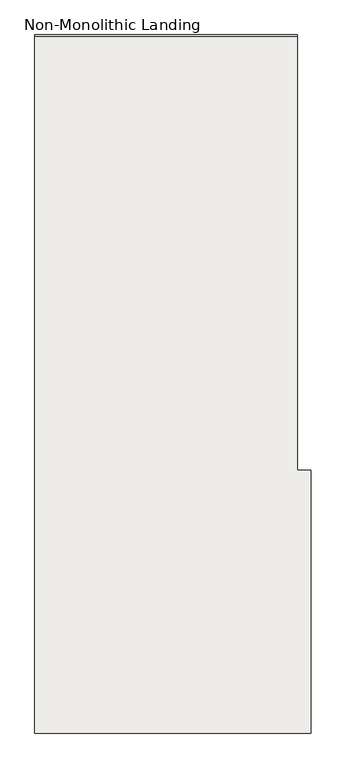
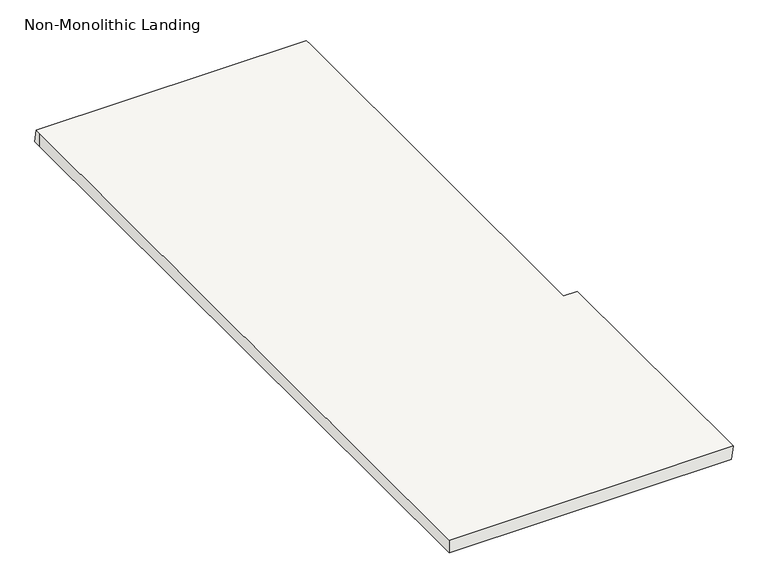
"""IFC4 building model written with IfcOpenShell, lengths in millimetres: slab geometry, Non-Monolithic Landing."""

from ifc_helpers import new_model, si_unit, origin, place, context, project, spatial, faceted_brep, source, transform, mapped, element, save


def non_monolithic_landing_de183352(model_context):
    return source(origin(), model_context, "Body", "Brep", [
        faceted_brep([(-11551.2529994, 5709.8660835, 1043.4782609), (-11602.0529994, 5709.8660835, 1043.4782609), (-11602.0529994, 7333.8660835, 1043.4782609), (-11602.0529994, 7358.8660835, 1043.4782609), (-12602.0787807, 7358.8660835, 1043.4782609), (-12602.0787807, 7333.8660835, 1043.4782609), (-12602.0787807, 4709.8403022, 1043.4782609), (-11551.2529994, 4709.8403022, 1043.4782609), (-11602.0529994, 7333.8660835, 993.4782609), (-11602.0529994, 5709.8660835, 993.4782609), (-11558.4404994, 5709.8660835, 993.4782609), (-11558.4404994, 4709.8403022, 993.4782609), (-12602.0787807, 4709.8403022, 993.4782609), (-12602.0787807, 7333.8660835, 993.4782609), (-12602.0787807, 7366.0535835, 993.4782609), (-11602.0529994, 7366.0535835, 993.4782609)], [[[0, 1, 2, 3, 4, 5, 6, 7]], [[8, 9, 10, 11, 12, 13, 14, 15]], [[1, 0, 10, 9]], [[6, 5, 13, 12]], [[7, 6, 12, 11]], [[0, 7, 11, 10]], [[3, 15, 14, 4]], [[2, 1, 9, 8]], [[3, 2, 8, 15]], [[5, 4, 14, 13]]]),
    ])


if __name__ == "__main__":
    model = new_model("IFC4")
    model_context = context("Model", 3, world=origin())
    ifc_project = project(units=[si_unit("LENGTHUNIT", "METRE", prefix="MILLI")], contexts=[model_context])
    site = spatial("IfcSite", under=ifc_project)
    building = spatial("IfcBuilding", under=site)
    placement = place(None, origin())
    non_monolithic_landing_shape = non_monolithic_landing_de183352(model_context)
    element("IfcSlab", 1, ObjectType="Non-Monolithic Landing", at=placement, inside=building, context=model_context, shape_type="MappedRepresentation", body=[
        mapped(non_monolithic_landing_shape, transform((0.0, 0.0, 0.0), x_axis=(1.0, 0.0, 0.0), y_axis=(0.0, 1.0, 0.0), z_axis=(0.0, 0.0, 1.0))),
    ])
    save(model, "model.ifc")
